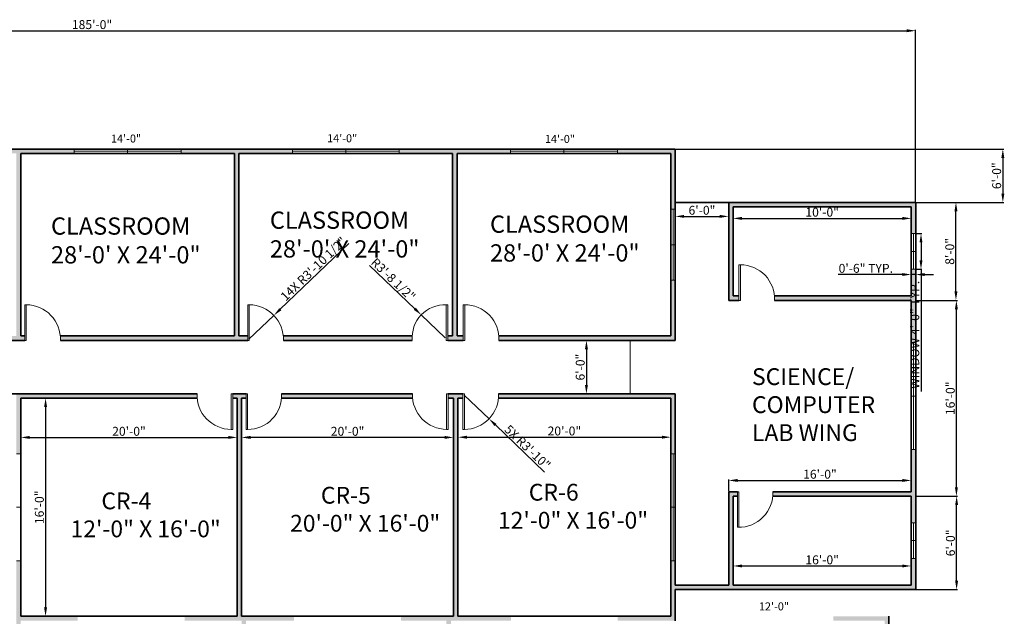
# Model space of a CAD drawing. Units: inches. Extents: x 2623 to 5095, y 1050 to 2384.
# Tile 4 of 4: x 3768 to 5095, y 1580 to 2384. Entities that reach past the tile are written whole.
import ezdxf

# ---------------------------------------------------------------- set-up
doc = ezdxf.new("R2010")
doc.units = ezdxf.units.IN
for name, color, linetype, lineweight in [('A-ANNO-DIMS', 2, 'Continuous', 13), ('A-ANNO-TEXT', 7, 'Continuous', 18), ('A-AREA-IDEN', 7, 'Continuous', 18), ('A-DOOR', 3, 'Continuous', 18), ('A-FLOR', 7, 'Continuous', 18), ('A-GLAZ', 4, 'Continuous', 18), ('A-WALL', 7, 'Continuous', 35)]:
    doc.layers.add(name, color=color, linetype=linetype, lineweight=lineweight)
doc.layers.add('A-WALL-PATT', color=251, linetype='Continuous', lineweight=9, true_color=0x636466)
doc.styles.get("Standard").update_dxf_attribs({"font": 'arial.ttf'})
doc.dimstyles.new('ISO-25', dxfattribs={"dimtxt": 12, "dimasz": 12, "dimexe": 1.25, "dimexo": 0.625, "dimtad": 1, "dimlunit": 3, "dimtxsty": 'Standard', "dimcen": 2.5, "dimadec": 0, "dimazin": 0, "dimtfac": 1, "dimtmove": 0, "dimatfit": 3, "dimfxl": 1, "dimarcsym": 0})

# ---------------------------------------------------------------- blocks, each defined once
blk = doc.blocks.new('*D18')
at = {"layer": 'A-ANNO-DIMS', "color": 0, "lineweight": -2, "transparency": 16777216}
for p, q in [((4976.3, 1741.6), (5032.1, 1741.6)), ((5030.9, 1627.6), (5030.9, 1729.6)), ((4976.3, 1615.6), (5032.1, 1615.6))]:
    blk.add_line(p, q, dxfattribs=at)
at = {"layer": 'A-ANNO-DIMS', "color": 0, "transparency": 16777216}
for points in [[(5028.9, 1729.6), (5032.9, 1729.6), (5030.9, 1741.6)], [(5028.9, 1627.6), (5032.9, 1627.6), (5030.9, 1615.6)]]:
    blk.add_solid(points, dxfattribs=at)
at = {"layer": 'Defpoints', "color": 0, "transparency": 16777216}
for p in [(4975.7, 1741.6), (5030.9, 1741.6), (4975.7, 1615.6)]:
    blk.add_point(p, dxfattribs=at)
at = {"layer": 'A-ANNO-DIMS', "color": 0, "transparency": 16777216, "insert": (5024.1, 1678.6), "char_height": 12, "attachment_point": 5, "rotation": 90}
blk.add_mtext('6\'-0"', dxfattribs=at)
blk = doc.blocks.new('*D19')
at = {"layer": 'A-ANNO-DIMS', "color": 0, "lineweight": -2, "transparency": 16777216}
for p, q in [((4976.3, 2005.6), (5031.9, 2005.6)), ((5030.6, 1753.6), (5030.6, 1993.6)), ((4976.3, 1741.6), (5031.9, 1741.6))]:
    blk.add_line(p, q, dxfattribs=at)
at = {"layer": 'A-ANNO-DIMS', "color": 0, "transparency": 16777216}
for points in [[(5028.6, 1993.6), (5032.6, 1993.6), (5030.6, 2005.6)], [(5028.6, 1753.6), (5032.6, 1753.6), (5030.6, 1741.6)]]:
    blk.add_solid(points, dxfattribs=at)
at = {"layer": 'Defpoints', "color": 0, "transparency": 16777216}
for p in [(4975.7, 2005.6), (5030.6, 2005.6), (4975.7, 1741.6)]:
    blk.add_point(p, dxfattribs=at)
at = {"layer": 'A-ANNO-DIMS', "color": 0, "transparency": 16777216, "insert": (5023.9, 1873.6), "char_height": 12, "attachment_point": 5, "rotation": 90}
blk.add_mtext('16\'-0"', dxfattribs=at)
blk = doc.blocks.new('*D20')
at = {"layer": 'A-ANNO-DIMS', "color": 0, "lineweight": -2, "transparency": 16777216}
for p, q in [((4976.3, 2137.6), (5031.2, 2137.6)), ((5030, 2017.6), (5030, 2125.6)), ((4976.3, 2005.6), (5031.2, 2005.6))]:
    blk.add_line(p, q, dxfattribs=at)
at = {"layer": 'A-ANNO-DIMS', "color": 0, "transparency": 16777216}
for points in [[(5028, 2125.6), (5032, 2125.6), (5030, 2137.6)], [(5028, 2017.6), (5032, 2017.6), (5030, 2005.6)]]:
    blk.add_solid(points, dxfattribs=at)
at = {"layer": 'Defpoints', "color": 0, "transparency": 16777216}
for p in [(4975.7, 2137.6), (5030, 2137.6), (4975.7, 2005.6)]:
    blk.add_point(p, dxfattribs=at)
at = {"layer": 'A-ANNO-DIMS', "color": 0, "transparency": 16777216, "insert": (5023.2, 2071.6), "char_height": 12, "attachment_point": 5, "rotation": 90}
blk.add_mtext('8\'-0"', dxfattribs=at)
blk = doc.blocks.new('*D21')
at = {"layer": 'A-ANNO-DIMS', "color": 0, "lineweight": -2, "transparency": 16777216}
for p, q in [((4651.7, 2137), (4651.7, 2117.5)), ((4723.7, 2137), (4723.7, 2117.5)), ((4663.7, 2118.8), (4711.7, 2118.8))]:
    blk.add_line(p, q, dxfattribs=at)
at = {"layer": 'A-ANNO-DIMS', "color": 0, "transparency": 16777216}
for points in [[(4663.7, 2120.8), (4663.7, 2116.8), (4651.7, 2118.8)], [(4711.7, 2120.8), (4711.7, 2116.8), (4723.7, 2118.8)]]:
    blk.add_solid(points, dxfattribs=at)
at = {"layer": 'Defpoints', "color": 0, "transparency": 16777216}
for p in [(4651.7, 2137.6), (4723.7, 2137.6), (4723.7, 2118.8)]:
    blk.add_point(p, dxfattribs=at)
at = {"layer": 'A-ANNO-DIMS', "color": 0, "transparency": 16777216, "insert": (4687.7, 2125.5), "char_height": 12, "attachment_point": 5}
blk.add_mtext('6\'-0"', dxfattribs=at)
blk = doc.blocks.new('*D31')
at = {"layer": 'A-ANNO-DIMS', "color": 0, "lineweight": -2, "transparency": 16777216}
for p, q in [((4729.7, 1622.2), (4729.7, 1648.7)), ((4741.7, 1647.5), (4957.7, 1647.5)), ((4969.7, 1622.2), (4969.7, 1648.7))]:
    blk.add_line(p, q, dxfattribs=at)
at = {"layer": 'A-ANNO-DIMS', "color": 0, "transparency": 16777216}
for points in [[(4741.7, 1649.5), (4741.7, 1645.5), (4729.7, 1647.5)], [(4957.7, 1649.5), (4957.7, 1645.5), (4969.7, 1647.5)]]:
    blk.add_solid(points, dxfattribs=at)
at = {"layer": 'Defpoints', "color": 0, "transparency": 16777216}
for p in [(4969.7, 1647.5), (4729.7, 1621.6), (4969.7, 1621.6)]:
    blk.add_point(p, dxfattribs=at)
at = {"layer": 'A-ANNO-DIMS', "color": 0, "transparency": 16777216, "insert": (4849.7, 1654.2), "char_height": 12, "attachment_point": 5}
blk.add_mtext('16\'-0"', dxfattribs=at)
blk = doc.blocks.new('*D32')
at = {"layer": 'A-ANNO-DIMS', "color": 0, "lineweight": -2, "transparency": 16777216}
for p, q in [((4723.7, 1748.2), (4723.7, 1764.1)), ((4735.7, 1762.8), (4957.7, 1762.8)), ((4969.7, 1748.2), (4969.7, 1764.1))]:
    blk.add_line(p, q, dxfattribs=at)
at = {"layer": 'A-ANNO-DIMS', "color": 0, "transparency": 16777216}
for points in [[(4735.7, 1764.8), (4735.7, 1760.8), (4723.7, 1762.8)], [(4957.7, 1764.8), (4957.7, 1760.8), (4969.7, 1762.8)]]:
    blk.add_solid(points, dxfattribs=at)
at = {"layer": 'Defpoints', "color": 0, "transparency": 16777216}
for p in [(4969.7, 1762.8), (4723.7, 1747.6), (4969.7, 1747.6)]:
    blk.add_point(p, dxfattribs=at)
at = {"layer": 'A-ANNO-DIMS', "color": 0, "transparency": 16777216, "insert": (4846.7, 1769.6), "char_height": 12, "attachment_point": 5}
blk.add_mtext('16\'-0"', dxfattribs=at)
blk = doc.blocks.new('*D33')
at = {"layer": 'A-ANNO-DIMS', "color": 0, "lineweight": -2, "transparency": 16777216}
for p, q in [((4729.7, 2131), (4729.7, 2114.9)), ((4969.7, 2131), (4969.7, 2114.9)), ((4741.7, 2116.1), (4957.7, 2116.1))]:
    blk.add_line(p, q, dxfattribs=at)
at = {"layer": 'A-ANNO-DIMS', "color": 0, "transparency": 16777216}
for points in [[(4741.7, 2118.1), (4741.7, 2114.1), (4729.7, 2116.1)], [(4957.7, 2118.1), (4957.7, 2114.1), (4969.7, 2116.1)]]:
    blk.add_solid(points, dxfattribs=at)
at = {"layer": 'Defpoints', "color": 0, "transparency": 16777216}
for p in [(4729.7, 2131.6), (4969.7, 2131.6), (4969.7, 2116.1)]:
    blk.add_point(p, dxfattribs=at)
at = {"layer": 'A-ANNO-DIMS', "color": 0, "transparency": 16777216, "insert": (4849.7, 2122.9), "char_height": 12, "attachment_point": 5}
blk.add_mtext('10\'-0"', dxfattribs=at)
blk = doc.blocks.new('*D34')
at = {"layer": 'A-ANNO-DIMS', "color": 0, "lineweight": -2, "transparency": 16777216}
for p, q in [((4651.1, 1951.6), (4530.7, 1951.6)), ((4532, 1939.6), (4532, 1891.6)), ((4651.1, 1879.6), (4530.7, 1879.6))]:
    blk.add_line(p, q, dxfattribs=at)
at = {"layer": 'A-ANNO-DIMS', "color": 0, "transparency": 16777216}
for points in [[(4530, 1939.6), (4534, 1939.6), (4532, 1951.6)], [(4530, 1891.6), (4534, 1891.6), (4532, 1879.6)]]:
    blk.add_solid(points, dxfattribs=at)
at = {"layer": 'Defpoints', "color": 0, "transparency": 16777216}
for p in [(4651.7, 1951.6), (4532, 1879.6), (4651.7, 1879.6)]:
    blk.add_point(p, dxfattribs=at)
at = {"layer": 'A-ANNO-DIMS', "color": 0, "transparency": 16777216, "insert": (4525.2, 1915.6), "char_height": 12, "attachment_point": 5, "rotation": 90}
blk.add_mtext('6\'-0"', dxfattribs=at)
blk = doc.blocks.new('*D35')
at = {"layer": 'A-ANNO-DIMS', "color": 0, "lineweight": -2, "transparency": 16777216}
for p, q in [((4358.9, 1873), (4358.9, 1819.9)), ((4645.7, 1873), (4645.7, 1819.9)), ((4370.9, 1821.1), (4633.7, 1821.1))]:
    blk.add_line(p, q, dxfattribs=at)
at = {"layer": 'A-ANNO-DIMS', "color": 0, "transparency": 16777216}
for points in [[(4370.9, 1823.1), (4370.9, 1819.1), (4358.9, 1821.1)], [(4633.7, 1823.1), (4633.7, 1819.1), (4645.7, 1821.1)]]:
    blk.add_solid(points, dxfattribs=at)
at = {"layer": 'Defpoints', "color": 0, "transparency": 16777216}
for p in [(4358.9, 1873.6), (4645.7, 1873.6), (4645.7, 1821.1)]:
    blk.add_point(p, dxfattribs=at)
at = {"layer": 'A-ANNO-DIMS', "color": 0, "transparency": 16777216, "insert": (4502.3, 1827.9), "char_height": 12, "attachment_point": 5}
blk.add_mtext('20\'-0"', dxfattribs=at)
blk = doc.blocks.new('*D36')
at = {"layer": 'A-ANNO-DIMS', "color": 0, "lineweight": -2, "transparency": 16777216}
for p, q in [((4067.3, 1873), (4067.3, 1819.5)), ((4352.9, 1873), (4352.9, 1819.5)), ((4340.9, 1820.8), (4079.3, 1820.8))]:
    blk.add_line(p, q, dxfattribs=at)
at = {"layer": 'A-ANNO-DIMS', "color": 0, "transparency": 16777216}
for points in [[(4079.3, 1822.8), (4079.3, 1818.8), (4067.3, 1820.8)], [(4340.9, 1822.8), (4340.9, 1818.8), (4352.9, 1820.8)]]:
    blk.add_solid(points, dxfattribs=at)
at = {"layer": 'Defpoints', "color": 0, "transparency": 16777216}
for p in [(4067.3, 1873.6), (4352.9, 1873.6), (4067.3, 1820.8)]:
    blk.add_point(p, dxfattribs=at)
at = {"layer": 'A-ANNO-DIMS', "color": 0, "transparency": 16777216, "insert": (4210.1, 1827.5), "char_height": 12, "attachment_point": 5}
blk.add_mtext('20\'-0"', dxfattribs=at)
blk = doc.blocks.new('*D37')
at = {"layer": 'A-ANNO-DIMS', "color": 0, "lineweight": -2, "transparency": 16777216}
for p, q in [((3769.7, 1873), (3769.7, 1819.5)), ((4061.3, 1873), (4061.3, 1819.5)), ((3781.7, 1820.8), (4049.3, 1820.8))]:
    blk.add_line(p, q, dxfattribs=at)
at = {"layer": 'A-ANNO-DIMS', "color": 0, "transparency": 16777216}
for points in [[(3781.7, 1822.8), (3781.7, 1818.8), (3769.7, 1820.8)], [(4049.3, 1822.8), (4049.3, 1818.8), (4061.3, 1820.8)]]:
    blk.add_solid(points, dxfattribs=at)
at = {"layer": 'Defpoints', "color": 0, "transparency": 16777216}
for p in [(3769.7, 1873.6), (4061.3, 1873.6), (4061.3, 1820.8)]:
    blk.add_point(p, dxfattribs=at)
at = {"layer": 'A-ANNO-DIMS', "color": 0, "transparency": 16777216, "insert": (3915.5, 1827.5), "char_height": 12, "attachment_point": 5}
blk.add_mtext('20\'-0"', dxfattribs=at)
blk = doc.blocks.new('*D38')
at = {"layer": 'A-ANNO-DIMS', "color": 0, "lineweight": -2, "transparency": 16777216}
for p, q in [((3770.3, 1873.6), (3804.3, 1873.6)), ((3803.1, 1861.6), (3803.1, 1591.6)), ((3770.3, 1579.6), (3804.3, 1579.6))]:
    blk.add_line(p, q, dxfattribs=at)
at = {"layer": 'A-ANNO-DIMS', "color": 0, "transparency": 16777216}
for points in [[(3801.1, 1861.6), (3805.1, 1861.6), (3803.1, 1873.6)], [(3801.1, 1591.6), (3805.1, 1591.6), (3803.1, 1579.6)]]:
    blk.add_solid(points, dxfattribs=at)
at = {"layer": 'Defpoints', "color": 0, "transparency": 16777216}
for p in [(3769.7, 1873.6), (3769.7, 1579.6), (3803.1, 1579.6)]:
    blk.add_point(p, dxfattribs=at)
at = {"layer": 'A-ANNO-DIMS', "color": 0, "transparency": 16777216, "insert": (3796.3, 1726.6), "char_height": 12, "attachment_point": 5, "rotation": 90}
blk.add_mtext('16\'-0"', dxfattribs=at)
blk = doc.blocks.new('WIN-144-DOUBLE-LIGHT')
for p, q in [((0, 6), (0, 0)), ((144, 3), (0, 3)), ((72, 6), (72, 0)), ((144, 6), (144, 0))]:
    blk.add_line(p, q)
blk = doc.blocks.new('WIN-96-DOUBLE-LIGHT')
for p, q in [((0, 6), (0, 0)), ((0, 3), (96, 3)), ((48, 6), (48, 0)), ((96, 6), (96, 0))]:
    blk.add_line(p, q)
blk = doc.blocks.new('WIN-48-DOUBLE-LIGHT')
for p, q in [((0, 48), (6, 48)), ((3, 48), (3, 0)), ((0, 24), (6, 24)), ((0, 0), (6, 0))]:
    blk.add_line(p, q)
blk = doc.blocks.new('DOOR-48-LEAF-AND-JAMBS')
for p, q in [((0, 48), (0, 0)), ((2, 48), (0, 48)), ((0, 48), (0, 42)), ((2, 0), (2, 48)), ((48, 48), (48, 42)), ((0, 0), (2, 0))]:
    blk.add_line(p, q)
blk = doc.blocks.new('*D57')
at = {"layer": 'A-ANNO-DIMS', "color": 0, "lineweight": -2, "transparency": 16777216}
for p, q in [((4976.3, 2095.6), (4984.2, 2095.6)), ((4982.9, 2083.6), (4982.9, 2059.6)), ((4976.3, 2047.6), (4984.2, 2047.6)), ((4982.9, 2047.6), (4982.9, 1882.5))]:
    blk.add_line(p, q, dxfattribs=at)
at = {"layer": 'A-ANNO-DIMS', "color": 0, "transparency": 16777216}
for points in [[(4980.9, 2083.6), (4984.9, 2083.6), (4982.9, 2095.6)], [(4980.9, 2059.6), (4984.9, 2059.6), (4982.9, 2047.6)]]:
    blk.add_solid(points, dxfattribs=at)
at = {"layer": 'Defpoints', "color": 0, "transparency": 16777216}
for p in [(4975.7, 2095.6), (4975.7, 2047.6), (4982.9, 2047.6)]:
    blk.add_point(p, dxfattribs=at)
at = {"layer": 'A-ANNO-DIMS', "color": 0, "transparency": 16777216, "insert": (4976.1, 1959.1), "char_height": 12, "attachment_point": 5, "rotation": 90}
blk.add_mtext('WINDOW 4\'-0" TYP.', dxfattribs=at)
blk = doc.blocks.new('*D58')
at = {"layer": 'A-ANNO-DIMS', "color": 0, "lineweight": -2, "transparency": 16777216}
for p, q in [((4969.7, 2047), (4969.7, 2039.2)), ((4975.7, 2047), (4975.7, 2039.2)), ((4957.7, 2040.4), (4871.3, 2040.4)), ((4975.7, 2040.4), (4969.7, 2040.4)), ((4987.7, 2040.4), (4999.7, 2040.4))]:
    blk.add_line(p, q, dxfattribs=at)
at = {"layer": 'A-ANNO-DIMS', "color": 0, "transparency": 16777216}
for points in [[(4957.7, 2042.4), (4957.7, 2038.4), (4969.7, 2040.4)], [(4987.7, 2042.4), (4987.7, 2038.4), (4975.7, 2040.4)]]:
    blk.add_solid(points, dxfattribs=at)
at = {"layer": 'Defpoints', "color": 0, "transparency": 16777216}
for p in [(4969.7, 2047.6), (4975.7, 2047.6), (4969.7, 2040.4)]:
    blk.add_point(p, dxfattribs=at)
at = {"layer": 'A-ANNO-DIMS', "color": 0, "transparency": 16777216, "insert": (4908.5, 2047.2), "char_height": 12, "attachment_point": 5}
blk.add_mtext('0\'-6" TYP.', dxfattribs=at)
blk = doc.blocks.new('*D65')
at = {"layer": 'A-ANNO-DIMS', "color": 0, "lineweight": -2, "transparency": 16777216}
for p, q in [((2755.7, 2252.2), (2755.7, 2370.3)), ((2767.7, 2369.1), (4963.7, 2369.1)), ((4975.7, 2138.2), (4975.7, 2370.3))]:
    blk.add_line(p, q, dxfattribs=at)
at = {"layer": 'A-ANNO-DIMS', "color": 0, "transparency": 16777216}
for points in [[(2767.7, 2371.1), (2767.7, 2367.1), (2755.7, 2369.1)], [(4963.7, 2371.1), (4963.7, 2367.1), (4975.7, 2369.1)]]:
    blk.add_solid(points, dxfattribs=at)
at = {"layer": 'Defpoints', "color": 0, "transparency": 16777216}
for p in [(4975.7, 2369.1), (2755.7, 2251.6), (4975.7, 2137.6)]:
    blk.add_point(p, dxfattribs=at)
at = {"layer": 'A-ANNO-DIMS', "color": 0, "transparency": 16777216, "insert": (3865.7, 2375.8), "char_height": 12, "attachment_point": 5}
blk.add_mtext('185\'-0"', dxfattribs=at)
blk = doc.blocks.new('*D67')
at = {"layer": 'A-ANNO-DIMS', "color": 0, "lineweight": -2, "transparency": 16777216}
for p, q in [((4652.3, 2209.6), (5094.4, 2209.6)), ((5093.2, 2197.6), (5093.2, 2149.6)), ((4976.3, 2137.6), (5094.4, 2137.6))]:
    blk.add_line(p, q, dxfattribs=at)
at = {"layer": 'A-ANNO-DIMS', "color": 0, "transparency": 16777216}
for points in [[(5091.2, 2197.6), (5095.2, 2197.6), (5093.2, 2209.6)], [(5091.2, 2149.6), (5095.2, 2149.6), (5093.2, 2137.6)]]:
    blk.add_solid(points, dxfattribs=at)
at = {"layer": 'Defpoints', "color": 0, "transparency": 16777216}
for p in [(4651.7, 2209.6), (4975.7, 2137.6), (5093.2, 2137.6)]:
    blk.add_point(p, dxfattribs=at)
at = {"layer": 'A-ANNO-DIMS', "color": 0, "transparency": 16777216, "insert": (5086.4, 2173.6), "char_height": 12, "attachment_point": 5, "rotation": 90}
blk.add_mtext('6\'-0"', dxfattribs=at)
blk = doc.blocks.new('*D71')
at = {"layer": 'A-ANNO-DIMS', "color": 0, "lineweight": -2, "transparency": 16777216}
for p, q in [((4211.8, 2082.1), (4119.4, 1993.6)), ((4077.2, 1953.1), (4110.8, 1985.3))]:
    blk.add_line(p, q, dxfattribs=at)
at = {"layer": 'A-ANNO-DIMS', "color": 0, "transparency": 16777216}
blk.add_solid([(4118, 1995), (4120.8, 1992.2), (4110.8, 1985.3)], dxfattribs=at)
at = {"layer": 'Defpoints', "color": 0, "transparency": 16777216}
for p in [(4110.8, 1985.3), (4077.2, 1953.1)]:
    blk.add_point(p, dxfattribs=at)
at = {"layer": 'A-ANNO-DIMS', "color": 0, "transparency": 16777216, "insert": (4165.2, 2046.9), "char_height": 12, "attachment_point": 5, "rotation": 43.7808}
blk.add_mtext('14X R3\'-10 1/2"', dxfattribs=at)
blk = doc.blocks.new('*D72')
at = {"layer": 'A-ANNO-DIMS', "color": 0, "lineweight": -2, "transparency": 16777216}
for p, q in [((4367.4, 1877.8), (4400.8, 1845.9)), ((4475.7, 1774.1), (4409.4, 1837.6))]:
    blk.add_line(p, q, dxfattribs=at)
at = {"layer": 'A-ANNO-DIMS', "color": 0, "transparency": 16777216}
blk.add_solid([(4410.8, 1839), (4408, 1836.1), (4400.8, 1845.9)], dxfattribs=at)
at = {"layer": 'Defpoints', "color": 0, "transparency": 16777216}
for p in [(4367.4, 1877.8), (4400.8, 1845.9)]:
    blk.add_point(p, dxfattribs=at)
at = {"layer": 'A-ANNO-DIMS', "color": 0, "transparency": 16777216, "insert": (4451.5, 1806.5), "char_height": 12, "attachment_point": 5, "rotation": 316.2194}
blk.add_mtext('5X R3\'-10"', dxfattribs=at)
blk = doc.blocks.new('*D75')
at = {"layer": 'A-ANNO-DIMS', "color": 0, "lineweight": -2, "transparency": 16777216}
for p, q in [((4239.7, 2052.8), (4300.7, 1994.2)), ((4341.6, 1955.1), (4309.4, 1985.9))]:
    blk.add_line(p, q, dxfattribs=at)
at = {"layer": 'A-ANNO-DIMS', "color": 0, "transparency": 16777216}
blk.add_solid([(4302.1, 1995.7), (4299.4, 1992.8), (4309.4, 1985.9)], dxfattribs=at)
at = {"layer": 'Defpoints', "color": 0, "transparency": 16777216}
for p in [(4309.4, 1985.9), (4341.6, 1955.1)]:
    blk.add_point(p, dxfattribs=at)
at = {"layer": 'A-ANNO-DIMS', "color": 0, "transparency": 16777216, "insert": (4270.6, 2032.6), "char_height": 12, "attachment_point": 5, "rotation": 316.2184}
blk.add_mtext('R3\'-8 1/2"', dxfattribs=at)

msp = doc.modelspace()

# ---------------------------------------------------------------- hatches: boundary and pattern name
at = {"layer": 'A-WALL-PATT'}
h = msp.add_hatch(color=256, dxfattribs=at)
h.dxf.hatch_style = 1
h.paths.add_polyline_path([(3103.717, 2251.615), (2755.717, 2251.615), (2755.717, 2173.615), (2761.717, 2173.615), (2761.717, 2245.615), (3097.717, 2245.615), (3097.717, 2015.688), (3100.811, 2015.688, -0.01561511), (3103.717, 2015.688)])
h.paths.add_polyline_path([(3103.717, 1967.688), (3097.717, 1967.688), (3097.717, 1957.615), (2761.717, 1957.615), (2761.717, 2029.615), (2755.717, 2029.615), (2755.717, 1915.615), (2761.717, 1915.615), (2761.717, 1951.615), (3097.717, 1951.615), (3097.717, 1943.747), (3103.717, 1943.747)])
h.paths.add_polyline_path([(3103.717, 1895.747, -0.01327118), (3101.235, 1895.747), (3097.717, 1895.747), (3097.717, 1735.615), (2761.717, 1735.615), (2761.717, 1771.615), (2755.717, 1771.615), (2755.717, 1693.615), (2761.717, 1693.615), (2761.717, 1729.615), (3097.717, 1729.615), (3097.717, 1721.81), (3103.717, 1721.81)])
h.paths.add_polyline_path([(2761.717, 1573.615), (2755.717, 1573.615), (2755.717, 1405.615), (2761.717, 1405.615)])
h.paths.add_polyline_path([(2761.717, 1285.615), (2755.717, 1285.615), (2755.717, 1243.615), (2857.717, 1243.615), (2857.717, 1249.615), (2761.717, 1249.615)])
h.paths.add_polyline_path([(3152.017, 1249.615), (3103.717, 1249.615), (3103.717, 1489.615), (3237.319, 1489.615, -0.03349431), (3237.344, 1495.615), (3103.717, 1495.615), (3103.717, 1507.046), (3097.717, 1507.046), (3097.717, 1249.615), (3001.717, 1249.615), (3001.717, 1243.615), (3103.717, 1243.615), (3152.017, 1243.615)])
h.paths.add_polyline_path([(3103.717, 1673.81, -0.01537929), (3100.853, 1673.81), (3097.717, 1673.81), (3097.717, 1555.046), (3101.163, 1555.046, -0.01366836), (3103.717, 1555.046)])
h.paths.add_polyline_path([(3302.317, 1249.615), (3302.317, 1297.615), (3385.117, 1297.615), (3385.117, 1303.615), (3302.317, 1303.615), (3302.317, 1489.615), (3503.954, 1489.615), (3503.954, 1492.911, -0.01449155), (3503.954, 1495.615), (3285.344, 1495.615), (3285.344, 1489.615), (3296.317, 1489.615), (3296.317, 1249.615), (3248.017, 1249.615), (3248.017, 1243.615), (3302.317, 1243.615)])
h.paths.add_polyline_path([(3569.917, 1489.615), (3579.094, 1489.615), (3579.094, 1495.615), (3551.954, 1495.615), (3551.954, 1489.615), (3563.917, 1489.615), (3563.917, 1303.615), (3481.117, 1303.615), (3481.117, 1297.615), (3563.917, 1297.615), (3563.917, 1249.615), (3563.917, 1243.615), (3618.817, 1243.615), (3618.817, 1249.615), (3569.917, 1249.615)])
h.paths.add_polyline_path([(3846.517, 1249.615), (3769.717, 1249.615), (3769.717, 1573.615), (3846.517, 1573.615), (3846.517, 1579.615), (3769.717, 1579.615), (3769.717, 1654.615), (3763.717, 1654.615), (3763.717, 1495.615), (3627.094, 1495.615, -0.01677945), (3627.094, 1492.499), (3627.094, 1489.615), (3763.717, 1489.615), (3763.717, 1249.615), (3714.817, 1249.615), (3714.817, 1243.615), (3763.717, 1243.615), (3846.517, 1243.615)])
h.paths.add_polyline_path([(4084.941, 1249.615), (4073.317, 1249.615), (4073.317, 1305.13), (4067.317, 1305.13), (4067.317, 1249.615), (3990.517, 1249.615), (3990.517, 1243.615), (4084.941, 1243.615)])
h.paths.add_polyline_path([(4277.411, 1249.615), (4208.317, 1249.615), (4208.317, 1366.615), (4282.724, 1366.615), (4282.724, 1370.675, -0.01031167), (4282.724, 1372.615), (4115.317, 1372.615), (4115.317, 1381.792), (4114.62, 1381.792, -0.02925374), (4109.317, 1381.792), (4109.317, 1372.615), (4073.317, 1372.615), (4067.317, 1372.615), (4067.317, 1353.13), (4073.317, 1353.13), (4073.317, 1366.615), (4202.317, 1366.615), (4202.317, 1249.615), (4120.941, 1249.615), (4120.941, 1243.615), (4277.411, 1243.615)])
h.paths.add_polyline_path([(4939.717, 1300.615), (4933.717, 1300.615), (4818.498, 1300.615), (4818.498, 1294.615), (4933.717, 1294.615), (4933.717, 1249.615), (4349.317, 1249.615), (4349.317, 1294.615), (4465.249, 1294.615), (4465.249, 1300.615), (4349.317, 1300.615), (4349.317, 1573.615), (4430.317, 1573.615), (4430.317, 1579.615), (4358.917, 1579.615), (4358.917, 1873.615), (4365.566, 1873.615), (4365.566, 1879.615), (4345.539, 1879.615), (4345.539, 1873.615), (4352.917, 1873.615), (4352.917, 1579.615), (4282.117, 1579.615), (4282.117, 1573.615), (4343.317, 1573.615), (4343.317, 1456.615), (4177.166, 1456.615), (4177.166, 1450.615), (4343.317, 1450.615), (4343.317, 1372.615), (4330.724, 1372.615), (4330.724, 1366.615), (4343.317, 1366.615), (4343.317, 1249.615), (4313.411, 1249.615), (4313.411, 1243.615), (4939.717, 1243.615)])
h = msp.add_hatch(color=256, dxfattribs=at)
h.dxf.hatch_style = 1
h.paths.add_polyline_path([(4651.717, 1615.615), (4975.717, 1615.615), (4975.717, 1657.615), (4969.717, 1657.615), (4969.717, 1621.615), (4729.717, 1621.615), (4729.717, 1741.615), (4735.396, 1741.615), (4735.396, 1747.615), (4723.717, 1747.615), (4723.717, 1621.615), (4651.717, 1621.615), (4651.717, 1654.615), (4645.717, 1654.615), (4645.717, 1579.615), (4574.317, 1579.615), (4574.317, 1573.615), (4651.717, 1573.615)])
h.paths.add_polyline_path([(4939.717, 1579.615), (4864.717, 1579.615), (4864.717, 1573.615), (4933.717, 1573.615), (4933.717, 1345.615), (4939.717, 1345.615)])
h.paths.add_polyline_path([(4975.717, 1804.615), (4969.717, 1804.615), (4969.717, 1747.615), (4783.396, 1747.615, -0.01744529), (4783.396, 1744.379), (4783.396, 1741.615), (4969.717, 1741.615), (4969.717, 1705.615), (4975.717, 1705.615)])
h.paths.add_polyline_path([(4975.717, 2047.615), (4969.717, 2047.615), (4969.717, 2011.615), (4785.608, 2011.615), (4785.608, 2008.9, -0.01771988), (4785.608, 2005.615), (4969.717, 2005.615), (4969.717, 1948.615), (4975.717, 1948.615), (4975.717, 2005.615)])
h.paths.add_polyline_path([(4975.717, 2137.615), (4729.717, 2137.615), (4723.717, 2137.615), (4723.717, 2005.615), (4737.608, 2005.615), (4737.608, 2011.615), (4729.717, 2011.615), (4729.717, 2131.615), (4969.717, 2131.615), (4969.717, 2095.615), (4975.717, 2095.615)])
h.paths.add_polyline_path([(4651.717, 2209.615), (4573.717, 2209.615), (4573.717, 2203.615), (4645.717, 2203.615), (4645.717, 2128.615), (4651.717, 2128.615)])
h.paths.add_polyline_path([(4651.717, 2032.615), (4645.717, 2032.615), (4645.717, 1957.615), (4413.911, 1957.615), (4413.911, 1956.398, -0.02623296), (4413.911, 1951.615), (4651.717, 1951.615)])
h.paths.add_polyline_path([(4357.717, 2203.615), (4429.717, 2203.615), (4429.717, 2209.615), (4279.717, 2209.615), (4279.717, 2203.615), (4351.717, 2203.615), (4351.717, 1957.615), (4345.154, 1957.615), (4345.154, 1951.615), (4365.911, 1951.615), (4365.911, 1957.615), (4357.717, 1957.615)])
h.paths.add_polyline_path([(4063.717, 2203.615), (4135.717, 2203.615), (4135.717, 2209.615), (3985.717, 2209.615), (3985.717, 2203.615), (4057.717, 2203.615), (4057.717, 1957.615), (3823.079, 1957.615), (3823.079, 1955.024, -0.01841239), (3823.079, 1951.615), (4075.656, 1951.615), (4075.656, 1957.615), (4063.717, 1957.615)])
h.paths.add_polyline_path([(4297.09, 1957.615), (4123.656, 1957.615), (4123.656, 1954.68, -0.01649439), (4123.656, 1951.615), (4297.154, 1951.615, -0.03370804)])
h.paths.add_polyline_path([(3769.717, 2203.615), (3841.717, 2203.615), (3841.717, 2209.615), (3691.717, 2209.615), (3691.717, 2203.615), (3763.717, 2203.615), (3763.717, 1957.615), (3754.594, 1957.615), (3754.594, 1951.615), (3775.079, 1951.615), (3775.079, 1957.615), (3769.717, 1957.615)])
h.paths.add_polyline_path([(3706.594, 1957.102), (3706.594, 1957.615), (3529.616, 1957.615), (3529.616, 1955.888, -0.02330465), (3529.616, 1951.615), (3706.594, 1951.615, -0.03033114)])
h.paths.add_polyline_path([(3481.616, 1957.615), (3475.717, 1957.615), (3475.717, 2203.615), (3547.717, 2203.615), (3547.717, 2209.615), (3397.717, 2209.615), (3397.717, 2203.615), (3469.717, 2203.615), (3469.717, 1957.615), (3457.307, 1957.615), (3457.307, 1951.615), (3481.616, 1951.615)])
h.paths.add_polyline_path([(3409.307, 1954.491), (3409.307, 1957.615), (3181.717, 1957.615), (3181.717, 2203.615), (3253.717, 2203.615), (3253.717, 2209.615), (3175.717, 2209.615), (3175.717, 1747.615, -0.01406848), (3178.344, 1747.615), (3181.717, 1747.615), (3181.717, 1873.615), (3434.065, 1873.615), (3434.065, 1877.049, -0.01373428), (3434.065, 1879.615), (3181.717, 1879.615), (3181.717, 1951.615), (3409.307, 1951.615, -0.01544691)])
h.paths.add_polyline_path([(4651.717, 1879.615), (4413.566, 1879.615, -0.01934194), (4413.566, 1876.041), (4413.566, 1873.615), (4645.717, 1873.615), (4645.717, 1798.615), (4651.717, 1798.615)])
h.paths.add_polyline_path([(4138.117, 1579.615), (4067.317, 1579.615), (4067.317, 1873.615), (4073.262, 1873.615), (4073.262, 1879.615), (4055.249, 1879.615), (4055.249, 1873.615), (4061.317, 1873.615), (4061.317, 1579.615), (3990.517, 1579.615), (3990.517, 1573.615), (4067.317, 1573.615), (4067.317, 1450.615), (4109.317, 1450.615), (4109.317, 1429.792), (4115.317, 1429.792), (4115.317, 1450.615), (4129.166, 1450.615), (4129.166, 1456.615), (4073.317, 1456.615), (4073.317, 1573.615), (4138.117, 1573.615)])
h.paths.add_polyline_path([(4297.539, 1879.615), (4121.262, 1879.615, -0.02641892), (4121.262, 1874.8), (4121.262, 1873.615), (4297.539, 1873.615), (4297.539, 1876.326, -0.01774472)])
h.paths.add_polyline_path([(4007.249, 1879.615), (3763.717, 1879.615), (3763.717, 1798.615), (3769.717, 1798.615), (3769.717, 1873.615), (4007.249, 1873.615), (4007.249, 1876.064, -0.01921077)])
h.paths.add_polyline_path([(3715.717, 1573.615), (3469.717, 1573.615), (3469.717, 1567.615), (3715.717, 1567.615)])
h.paths.add_polyline_path([(3421.717, 1570.87), (3421.717, 1573.615), (3181.717, 1573.615), (3181.717, 1699.615), (3175.717, 1699.615), (3175.717, 1567.615), (3421.717, 1567.615, -0.01755055)])
h.paths.add_polyline_path([(3715.717, 1879.615), (3482.065, 1879.615), (3482.065, 1873.615), (3715.717, 1873.615)])

# ---------------------------------------------------------------- linework, layer by layer
at = {"layer": 'A-DOOR'}
for centre, radius, start, end in [((4739.278, 2007.257), 46.359, 357.969663, 89.592586), ((3776.814, 1953.319), 46.296, 357.890334, 89.671915), ((4077.211, 1953.148), 46.47, 358.110054, 89.452196), ((4341.572, 1955.09), 44.553, 87.963974, 184.473777), ((4368.362, 1954.006), 45.611, 356.994614, 90.567636), ((4053.44, 1877.84), 46.225, 177.798878, 269.763371), ((4075.73, 1877.208), 45.595, 269.411069, 3.026682), ((4343.867, 1877.97), 46.357, 177.966819, 269.595431), ((4367.387, 1877.828), 46.213, 270.221603, 2.216147), ((4737.038, 1745.997), 46.386, 269.207303, 1.99888)]:
    msp.add_arc(centre, radius, start, end, dxfattribs=at)
at = {"layer": 'A-FLOR'}
msp.add_line((4590.914, 1951.615), (4590.914, 1879.615), dxfattribs=at)
at = {"layer": 'A-GLAZ'}
for p, q in [((3769.717, 1798.615), (3763.717, 1798.615)), ((4645.717, 1798.615), (4651.717, 1798.615)), ((3769.717, 1726.615), (3763.717, 1726.615)), ((4969.717, 1705.615), (4975.717, 1705.615)), ((3769.717, 1654.615), (3763.717, 1654.615))]:
    msp.add_line(p, q, dxfattribs=at)
at = {"layer": 'A-WALL'}
for p, q in [((3175.717, 2209.615), (4651.717, 2209.615)), ((3769.717, 2203.615), (3769.717, 1957.615)), ((3769.717, 2203.615), (4057.717, 2203.615)), ((4057.717, 2203.615), (4057.717, 1957.615)), ((4063.717, 2203.615), (4063.717, 1957.615)), ((4063.717, 2203.615), (4351.717, 2203.615)), ((4351.717, 2203.615), (4351.717, 1957.615)), ((4357.717, 2203.615), (4357.717, 1957.615)), ((4357.717, 2203.615), (4645.717, 2203.615)), ((4645.717, 2203.615), (4645.717, 1957.615)), ((4651.717, 2209.615), (4651.717, 1951.615)), ((4651.717, 2137.615), (4729.717, 2137.615)), ((4723.717, 2137.615), (4723.717, 2005.615)), ((4729.717, 2137.615), (4975.717, 2137.615)), ((4975.717, 2137.615), (4975.717, 1951.615)), ((4729.717, 2131.615), (4729.717, 2011.615)), ((4729.717, 2131.615), (4969.717, 2131.615)), ((4969.717, 2131.615), (4969.717, 2011.615)), ((4723.717, 2005.615), (4737.608, 2005.615)), ((4729.717, 2011.615), (4737.608, 2011.615)), ((4785.608, 2011.615), (4969.717, 2011.615)), ((4785.608, 2005.615), (4969.717, 2005.615)), ((4969.717, 2005.615), (4969.717, 1747.615)), ((4975.717, 2005.615), (4975.717, 1615.615)), ((3754.594, 1951.615), (3775.079, 1951.615)), ((3769.717, 1957.615), (3775.079, 1957.615)), ((3823.079, 1957.615), (4057.717, 1957.615)), ((3823.079, 1951.615), (4075.656, 1951.615)), ((4063.717, 1957.615), (4075.656, 1957.615)), ((4123.656, 1957.615), (4297.154, 1957.615)), ((4123.656, 1951.615), (4297.154, 1951.615)), ((4345.154, 1957.615), (4351.717, 1957.615)), ((4345.154, 1951.615), (4365.911, 1951.615)), ((4357.717, 1957.615), (4365.911, 1957.615)), ((4413.911, 1957.615), (4645.717, 1957.615)), ((4413.911, 1951.615), (4651.717, 1951.615)), ((3482.065, 1879.615), (4007.249, 1879.615)), ((3769.717, 1873.615), (3769.717, 1579.615)), ((3769.717, 1873.615), (4007.249, 1873.615)), ((4055.249, 1879.615), (4073.262, 1879.615)), ((4055.249, 1873.615), (4061.317, 1873.615)), ((4061.317, 1873.615), (4061.317, 1579.615)), ((4067.317, 1873.615), (4067.317, 1579.615)), ((4067.317, 1873.615), (4073.262, 1873.615)), ((4121.262, 1879.615), (4297.539, 1879.615)), ((4121.262, 1873.615), (4297.539, 1873.615)), ((4345.539, 1879.615), (4365.566, 1879.615)), ((4345.539, 1873.615), (4352.917, 1873.615)), ((4352.917, 1873.615), (4352.917, 1579.615)), ((4358.917, 1873.615), (4358.917, 1579.615)), ((4358.917, 1873.615), (4365.566, 1873.615)), ((4413.566, 1879.615), (4651.717, 1879.615)), ((4413.566, 1873.615), (4645.717, 1873.615)), ((4645.717, 1873.615), (4645.717, 1579.615)), ((4651.717, 1879.615), (4651.717, 1621.615)), ((4723.717, 1747.615), (4735.396, 1747.615)), ((4723.717, 1747.615), (4723.717, 1621.615)), ((4729.717, 1741.615), (4735.396, 1741.615)), ((4729.717, 1741.615), (4729.717, 1621.615)), ((4783.396, 1747.615), (4969.717, 1747.615)), ((4783.396, 1741.615), (4969.717, 1741.615)), ((4969.717, 1741.615), (4969.717, 1621.615)), ((4651.717, 1621.615), (4723.717, 1621.615)), ((4729.717, 1621.615), (4969.717, 1621.615)), ((4651.717, 1615.615), (4975.717, 1615.615)), ((4651.717, 1615.615), (4651.717, 1573.615)), ((3769.717, 1579.615), (4061.317, 1579.615)), ((4067.317, 1579.615), (4352.917, 1579.615)), ((4358.917, 1579.615), (4645.717, 1579.615)), ((4939.717, 1579.615), (4939.717, 1243.615))]:
    msp.add_line(p, q, dxfattribs=at)

# ---------------------------------------------------------------- block references
at = {"layer": 'A-DOOR', "extrusion": (0, 0, -1), "zscale": -1, "rotation": 180}
for p in [(-4737.608, 2053.615), (-3775.079, 1999.615), (-4075.656, 1999.615), (-4365.911, 1999.615)]:
    msp.add_blockref('DOOR-48-LEAF-AND-JAMBS', p, dxfattribs=at)
at = {"layer": 'A-DOOR', "rotation": 180}
msp.add_blockref('DOOR-48-LEAF-AND-JAMBS', (4345.154, 1999.615), dxfattribs=at)
at = {"layer": 'A-DOOR', "extrusion": (0, 0, -1), "zscale": -1}
for p in [(-4055.249, 1831.615), (-4345.539, 1831.615)]:
    msp.add_blockref('DOOR-48-LEAF-AND-JAMBS', p, dxfattribs=at)
at = {"layer": 'A-DOOR'}
for p in [(4073.262, 1831.615), (4365.566, 1831.615), (4735.396, 1699.615)]:
    msp.add_blockref('DOOR-48-LEAF-AND-JAMBS', p, dxfattribs=at)
at = {"layer": 'A-GLAZ'}
for name, p, rotation in [('WIN-144-DOUBLE-LIGHT', (3985.717, 2209.615), 180), ('WIN-144-DOUBLE-LIGHT', (4279.717, 2209.615), 180), ('WIN-96-DOUBLE-LIGHT', (4651.717, 2032.615), 90.0000000000016), ('WIN-48-DOUBLE-LIGHT', (4975.717, 2095.615), 180), ('WIN-144-DOUBLE-LIGHT', (4975.717, 1804.615), 89.999999999998), ('WIN-144-DOUBLE-LIGHT', (4651.717, 1654.615), 90.00000000000018)]:
    msp.add_blockref(name, p, dxfattribs=dict(at, rotation=rotation))
for name, p in [('WIN-144-DOUBLE-LIGHT', (4429.717, 2203.615)), ('WIN-48-DOUBLE-LIGHT', (4969.717, 1657.615))]:
    msp.add_blockref(name, p, dxfattribs=at)

# ---------------------------------------------------------------- texts
at = {"layer": 'A-ANNO-TEXT', "char_height": 10.7617, "attachment_point": 1}
for s, insert in [('14\'-0"', (3891.311, 2229.153)), ('14\'-0"', (4182.506, 2229.484)), ('14\'-0"', (4476.002, 2228.61)), ('12\'-0"', (4764.456, 1598.365))]:
    msp.add_mtext_dynamic_manual_height_columns(s, width=391.78395, gutter_width=53.809, heights=[0], dxfattribs=dict(at, insert=insert))
at = {"layer": 'A-AREA-IDEN', "attachment_point": 1}
for s, width, gutter_width, insert, char_height in [('CLASSROOM\\P28\'-0\' X 24\'-0"', 847.02168, 116.332, (4105.396, 2125.356), 23.26647), ('CLASSROOM\\P28\'-0\' X 24\'-0"', 847.02168, 116.332, (3810.413, 2117.408), 23.26647), ('CLASSROOM\\P28\'-0\' X 24\'-0"', 847.02168, 116.332, (4402.05, 2119.944), 23.26647), ('SCIENCE/\\PCOMPUTER\\PLAB WING ', 824.72693, 113.27, (4755.13, 1914.067), 22.6541), ('      CR-5\\P20\'-0" X 16\'-0"', 824.72693, 113.27, (4132.619, 1754.182), 22.65406), ('      CR-6\\P12\'-0" X 16\'-0"', 824.72693, 113.27, (4412.764, 1758.231), 22.65406), ('      CR-4\\P12\'-0" X 16\'-0"', 824.72693, 113.27, (3836.778, 1746.59), 22.65406)]:
    msp.add_mtext_dynamic_manual_height_columns(s, width=width, gutter_width=gutter_width, heights=[0], dxfattribs=dict(at, insert=insert, char_height=char_height))

# ---------------------------------------------------------------- dimensions: what is measured, and where the dimension line sits
at = {"layer": 'A-ANNO-DIMS'}
dim = msp.add_linear_dim(base=(4975.717, 2369.065), p1=(2755.717, 2251.615), p2=(4975.717, 2137.615), dimstyle='ISO-25', override={"dimdec": 1, "dimlfac": 1, "dimrnd": 0, "dimzin": 1, "dimdsep": 46, "dimlunit": 4, "dimfrac": 2}, dxfattribs=at)
dim.commit()
dim.dimension.update_dxf_attribs({"geometry": '*D65', "text_midpoint": (3865.717, 2375.817)})
dim = msp.add_linear_dim(base=(5093.167, 2137.615), p1=(4651.717, 2209.615), p2=(4975.717, 2137.615), angle=90, dimstyle='ISO-25', override={"dimdec": 1, "dimlfac": 1, "dimrnd": 0, "dimzin": 1, "dimdsep": 46, "dimlunit": 4, "dimfrac": 2}, dxfattribs=at)
dim.commit()
dim.dimension.update_dxf_attribs({"geometry": '*D67', "text_midpoint": (5086.416, 2173.615)})
for base, p1, p2, text, picture, middle in [((4723.717, 2118.768), (4651.717, 2137.615), (4723.717, 2137.615), '6\'-0"', '*D21', (4687.717, 2125.52)), ((4969.717, 2116.125), (4729.717, 2131.615), (4969.717, 2131.615), '10\'-0"', '*D33', (4849.717, 2122.877)), ((4061.317, 1820.787), (3769.717, 1873.615), (4061.317, 1873.615), '20\'-0"', '*D37', (3915.517, 1827.538)), ((4067.317, 1820.789), (4352.917, 1873.615), (4067.317, 1873.615), '20\'-0"', '*D36', (4210.117, 1827.541)), ((4645.717, 1821.114), (4358.917, 1873.615), (4645.717, 1873.615), '20\'-0"', '*D35', (4502.317, 1827.866)), ((4969.717, 1762.812), (4723.717, 1747.615), (4969.717, 1747.615), '16\'-0"', '*D32', (4846.717, 1769.564)), ((4969.717, 1647.487), (4729.717, 1621.615), (4969.717, 1621.615), '16\'-0"', '*D31', (4849.717, 1654.239))]:
    dim = msp.add_linear_dim(base=base, p1=p1, p2=p2, text=text, dimstyle='ISO-25', override={"dimclrd": 0, "dimclre": 0, "dimclrt": 0}, dxfattribs=at)
    dim.commit()
    dim.dimension.update_dxf_attribs({"geometry": picture, "text_midpoint": middle})
for base, p1, p2, angle, text, override, picture, middle in [((5029.953, 2137.615), (4975.717, 2005.615), (4975.717, 2137.615), 90, '8\'-0"', {"dimclrd": 0, "dimclre": 0, "dimclrt": 0}, '*D20', (5023.202, 2071.615)), ((4982.917, 2047.615), (4975.717, 2095.615), (4975.717, 2047.615), 270, 'WINDOW <> TYP.', {"dimdec": 1, "dimlfac": 1, "dimrnd": 0, "dimzin": 1, "dimdsep": 46, "dimlunit": 4, "dimfrac": 2}, '*D57', (4976.084, 1959.065)), ((4969.717, 2040.415), (4975.717, 2047.615), (4969.717, 2047.615), 180, '<> TYP.', {"dimdec": 1, "dimlfac": 1, "dimrnd": 0, "dimzin": 1, "dimdsep": 46, "dimlunit": 4, "dimfrac": 2}, '*D58', (4908.519, 2047.167)), ((5030.626, 2005.615), (4975.717, 1741.615), (4975.717, 2005.615), 90, '16\'-0"', {"dimclrd": 0, "dimclre": 0, "dimclrt": 0}, '*D19', (5023.874, 1873.615)), ((4531.985, 1879.615), (4651.717, 1951.615), (4651.717, 1879.615), 90, '6\'-0"', {"dimclrd": 0, "dimclre": 0, "dimclrt": 0}, '*D34', (4525.233, 1915.615)), ((3803.083, 1579.615), (3769.717, 1873.615), (3769.717, 1579.615), 90, '16\'-0"', {"dimclrd": 0, "dimclre": 0, "dimclrt": 0}, '*D38', (3796.331, 1726.615)), ((5030.886, 1741.615), (4975.717, 1615.615), (4975.717, 1741.615), 90, '6\'-0"', {"dimclrd": 0, "dimclre": 0, "dimclrt": 0}, '*D18', (5024.134, 1678.615))]:
    dim = msp.add_linear_dim(base=base, p1=p1, p2=p2, angle=angle, text=text, dimstyle='ISO-25', override=override, dxfattribs=at)
    dim.commit()
    dim.dimension.update_dxf_attribs({"geometry": picture, "text_midpoint": middle})
for center, mpoint, text, picture, middle in [((4077.211, 1953.148), (4110.762, 1985.3), '14X <>', '*D71', (4165.2, 2046.934)), ((4367.387, 1877.828), (4400.753, 1845.853), '5X <>', '*D72', (4451.542, 1806.539))]:
    dim = msp.add_radius_dim(center=center, mpoint=mpoint, text=text, dimstyle='ISO-25', override={"dimdec": 1, "dimlfac": 1, "dimrnd": 0, "dimzin": 1, "dimdsep": 46, "dimlunit": 4, "dimfrac": 2}, dxfattribs=at)
    dim.commit()
    dim.dimension.update_dxf_attribs({"geometry": picture, "text_midpoint": middle})
dim = msp.add_radius_dim(center=(4341.572, 1955.09), mpoint=(4309.405, 1985.917), dimstyle='ISO-25', override={"dimdec": 1, "dimlfac": 1, "dimrnd": 0, "dimzin": 1, "dimdsep": 46, "dimlunit": 4, "dimfrac": 2}, dxfattribs=at)
dim.commit()
dim.dimension.update_dxf_attribs({"geometry": '*D75', "text_midpoint": (4270.6, 2032.571)})

doc.saveas('drawing.dxf')
